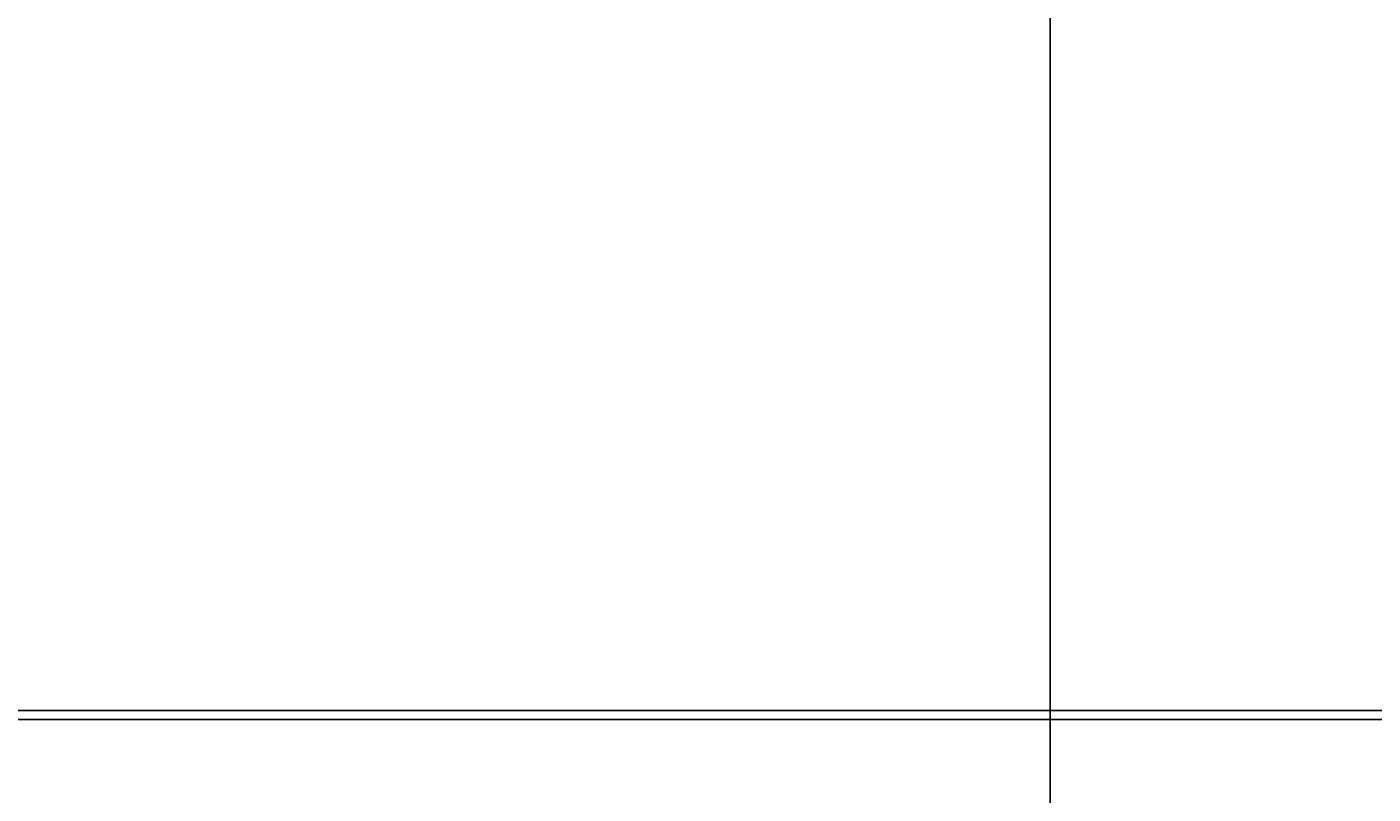
# Model space of a CAD drawing. Units: inches. Extents: x 35362 to 73946, y 43607 to 67532.
# Tile 93 of 134: x 49302 to 50119, y 49269 to 49735. Entities that reach past the tile are written whole.
import ezdxf

# ---------------------------------------------------------------- set-up
doc = ezdxf.new("R2010")
doc.units = ezdxf.units.IN
doc.header["$MEASUREMENT"] = 0
doc.layers.add('A-ANNO-DIMS', color=2, linetype='Continuous', lineweight=18)
doc.styles.get("Standard").update_dxf_attribs({"font": 'arial.ttf'})
doc.dimstyles.get("Standard").update_dxf_attribs({"dimtxt": 0.18, "dimasz": 0.18, "dimexe": 0.18, "dimexo": 0.0625, "dimgap": 0.09, "dimtad": 0, "dimtih": 1, "dimtoh": 1, "dimdec": 4, "dimzin": 0, "dimdsep": 46, "dimtxsty": 'Standard', "dimcen": 0.09, "dimadec": 0, "dimazin": 0, "dimtfac": 1, "dimtdec": 4, "dimtofl": 0, "dimtmove": 0, "dimatfit": 3, "dimfxl": 1, "dimtolj": 1, "dimtzin": 0, "dimarcsym": 0})

# ---------------------------------------------------------------- blocks, each defined once
blk = doc.blocks.new('*D11')
at = {"layer": 'A-ANNO-DIMS', "color": 0, "lineweight": -2, "transparency": 16777216}
for p, q in [((47978.66, 56028.77), (47978.66, 43606.68)), ((53109.76, 56028.77), (53109.76, 43606.68)), ((47978.84, 43606.86), (50543.87, 43606.86)), ((53109.58, 43606.86), (50544.55, 43606.86))]:
    blk.add_line(p, q, dxfattribs=at)
at = {"layer": 'A-ANNO-DIMS', "color": 0, "transparency": 16777216}
for points in [[(47978.84, 43606.89), (47978.84, 43606.83), (47978.66, 43606.86)], [(53109.58, 43606.89), (53109.58, 43606.83), (53109.76, 43606.86)]]:
    blk.add_solid(points, dxfattribs=at)
at = {"layer": 'Defpoints', "color": 0, "transparency": 16777216}
for p in [(47978.66, 56028.84), (53109.76, 56028.84), (53109.76, 43606.86)]:
    blk.add_point(p, dxfattribs=at)
at = {"layer": 'A-ANNO-DIMS', "color": 0, "transparency": 16777216, "insert": (50544.21, 43606.86), "char_height": 0.18, "attachment_point": 5}
blk.add_mtext('\\A1;5131', dxfattribs=at)
blk = doc.blocks.new('*D13')
at = {"layer": 'A-ANNO-DIMS', "color": 0, "lineweight": -2, "transparency": 16777216}
for p, q in [((48373.49, 51694.02), (48373.49, 43606.68)), ((51029.04, 51694.02), (51029.04, 43606.68)), ((48373.67, 43606.86), (49700.8, 43606.86)), ((51028.86, 43606.86), (49701.73, 43606.86))]:
    blk.add_line(p, q, dxfattribs=at)
at = {"layer": 'A-ANNO-DIMS', "color": 0, "transparency": 16777216}
for points in [[(48373.67, 43606.89), (48373.67, 43606.83), (48373.49, 43606.86)], [(51028.86, 43606.89), (51028.86, 43606.83), (51029.04, 43606.86)]]:
    blk.add_solid(points, dxfattribs=at)
at = {"layer": 'Defpoints', "color": 0, "transparency": 16777216}
for p in [(48373.49, 51694.09), (51029.04, 51694.09), (51029.04, 43606.86)]:
    blk.add_point(p, dxfattribs=at)
at = {"layer": 'A-ANNO-DIMS', "color": 0, "transparency": 16777216, "insert": (49701.27, 43606.86), "char_height": 0.18, "attachment_point": 5}
blk.add_mtext('\\A1;2655.6', dxfattribs=at)
blk = doc.blocks.new('*D17')
at = {"layer": 'A-ANNO-DIMS', "color": 0, "lineweight": -2, "transparency": 16777216}
for p, q in [((49923.31, 61293.22), (49923.31, 43606.68)), ((51913.93, 61293.22), (51913.93, 43606.68)), ((49923.49, 43606.86), (50918.16, 43606.86)), ((51913.75, 43606.86), (50919.07, 43606.86))]:
    blk.add_line(p, q, dxfattribs=at)
at = {"layer": 'A-ANNO-DIMS', "color": 0, "transparency": 16777216}
for points in [[(49923.49, 43606.89), (49923.49, 43606.83), (49923.31, 43606.86)], [(51913.75, 43606.89), (51913.75, 43606.83), (51913.93, 43606.86)]]:
    blk.add_solid(points, dxfattribs=at)
at = {"layer": 'Defpoints', "color": 0, "transparency": 16777216}
for p in [(49923.31, 61293.29), (51913.93, 61293.29), (51913.93, 43606.86)]:
    blk.add_point(p, dxfattribs=at)
at = {"layer": 'A-ANNO-DIMS', "color": 0, "transparency": 16777216, "insert": (50918.62, 43606.86), "char_height": 0.18, "attachment_point": 5}
blk.add_mtext('\\A1;1990.6', dxfattribs=at)
blk = doc.blocks.new('*D40')
at = {"layer": 'A-ANNO-DIMS', "color": 0, "lineweight": -2, "transparency": 16777216}
for p, q in [((56873.54, 53351.53), (35361.77, 53351.53)), ((35361.95, 53351.35), (35361.95, 51333.28)), ((35361.95, 49314.85), (35361.95, 51332.92)), ((51806.45, 49314.67), (35361.77, 49314.67))]:
    blk.add_line(p, q, dxfattribs=at)
at = {"layer": 'A-ANNO-DIMS', "color": 0, "transparency": 16777216}
for points in [[(35361.92, 53351.35), (35361.98, 53351.35), (35361.95, 53351.53)], [(35361.92, 49314.85), (35361.98, 49314.85), (35361.95, 49314.67)]]:
    blk.add_solid(points, dxfattribs=at)
at = {"layer": 'Defpoints', "color": 0, "transparency": 16777216}
for p in [(35361.95, 53351.53), (56873.6, 53351.53), (51806.52, 49314.67)]:
    blk.add_point(p, dxfattribs=at)
at = {"layer": 'A-ANNO-DIMS', "color": 0, "transparency": 16777216, "insert": (35361.95, 51333.1), "char_height": 0.18, "attachment_point": 5}
blk.add_mtext('\\A1;4036.9', dxfattribs=at)
blk = doc.blocks.new('*D67')
at = {"layer": 'A-ANNO-DIMS', "color": 0, "lineweight": -2, "transparency": 16777216}
for p, q in [((56873.54, 53351.53), (35361.77, 53351.53)), ((35361.95, 53351.35), (35361.95, 49400.89)), ((35361.95, 45450.07), (35361.95, 49400.53)), ((53793.58, 45449.89), (35361.77, 45449.89))]:
    blk.add_line(p, q, dxfattribs=at)
at = {"layer": 'A-ANNO-DIMS', "color": 0, "transparency": 16777216}
for points in [[(35361.92, 53351.35), (35361.98, 53351.35), (35361.95, 53351.53)], [(35361.92, 45450.07), (35361.98, 45450.07), (35361.95, 45449.89)]]:
    blk.add_solid(points, dxfattribs=at)
at = {"layer": 'Defpoints', "color": 0, "transparency": 16777216}
for p in [(35361.95, 53351.53), (56873.6, 53351.53), (53793.64, 45449.89)]:
    blk.add_point(p, dxfattribs=at)
at = {"layer": 'A-ANNO-DIMS', "color": 0, "transparency": 16777216, "insert": (35361.95, 49400.71), "char_height": 0.18, "attachment_point": 5}
blk.add_mtext('\\A1;7901.6', dxfattribs=at)
blk = doc.blocks.new('*D86')
at = {"layer": 'A-ANNO-DIMS', "color": 0, "lineweight": -2, "transparency": 16777216}
for p, q in [((51285.53, 49320.08), (35361.77, 49320.08)), ((35361.95, 49319.9), (35361.95, 49120.26)), ((35361.95, 48920.26), (35361.95, 49119.9)), ((51285.53, 48920.08), (35361.77, 48920.08))]:
    blk.add_line(p, q, dxfattribs=at)
at = {"layer": 'A-ANNO-DIMS', "color": 0, "transparency": 16777216}
for points in [[(35361.92, 49319.9), (35361.98, 49319.9), (35361.95, 49320.08)], [(35361.92, 48920.26), (35361.98, 48920.26), (35361.95, 48920.08)]]:
    blk.add_solid(points, dxfattribs=at)
at = {"layer": 'Defpoints', "color": 0, "transparency": 16777216}
for p in [(35361.95, 49320.08), (51285.59, 49320.08), (51285.59, 48920.08)]:
    blk.add_point(p, dxfattribs=at)
at = {"layer": 'A-ANNO-DIMS', "color": 0, "transparency": 16777216, "insert": (35361.95, 49120.08), "char_height": 0.18, "attachment_point": 5}
blk.add_mtext('\\A1;400.0', dxfattribs=at)

msp = doc.modelspace()

# ---------------------------------------------------------------- dimensions: what is measured, and where the dimension line sits
at = {"layer": 'A-ANNO-DIMS'}
for base, p1, p2, override, picture, middle in [((51913.931, 43606.859), (49923.307, 61293.286), (51913.931, 61293.286), {"dimdec": 1, "dimlfac": 1, "dimrnd": 0, "dimzin": 0, "dimdsep": 46, "dimlunit": 2}, '*D17', (50918.619, 43606.859)), ((53109.76, 43606.859), (47978.665, 56028.836), (53109.76, 56028.836), {"dimdec": 0, "dimlfac": 1, "dimrnd": 0, "dimzin": 0, "dimdsep": 46, "dimlunit": 2}, '*D11', (50544.212, 43606.859)), ((51029.043, 43606.859), (48373.492, 51694.087), (51029.043, 51694.087), {"dimdec": 1, "dimlfac": 1, "dimrnd": 0, "dimzin": 0, "dimdsep": 46, "dimlunit": 2}, '*D13', (49701.267, 43606.859))]:
    dim = msp.add_linear_dim(base=base, p1=p1, p2=p2, dimstyle='Standard', override=override, dxfattribs=at)
    dim.commit()
    dim.dimension.update_dxf_attribs({"geometry": picture, "text_midpoint": middle})
for base, p1, p2, picture, middle in [((35361.949, 53351.529), (51806.517, 49314.669), (56873.602, 53351.529), '*D40', (35361.949, 51333.099)), ((35361.949, 53351.529), (53793.638, 45449.894), (56873.602, 53351.529), '*D67', (35361.949, 49400.712)), ((35361.949, 49320.079), (51285.595, 48920.079), (51285.595, 49320.079), '*D86', (35361.949, 49120.079))]:
    dim = msp.add_linear_dim(base=base, p1=p1, p2=p2, angle=90, dimstyle='Standard', override={"dimdec": 1, "dimlfac": 1, "dimrnd": 0, "dimzin": 0, "dimdsep": 46, "dimlunit": 2}, dxfattribs=at)
    dim.commit()
    dim.dimension.update_dxf_attribs({"geometry": picture, "text_midpoint": middle})

doc.saveas('drawing.dxf')
